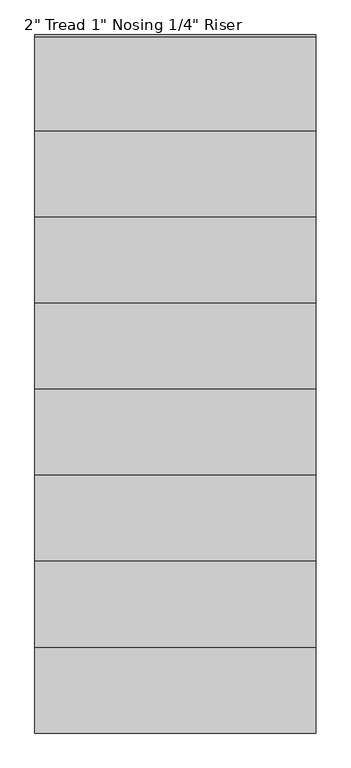
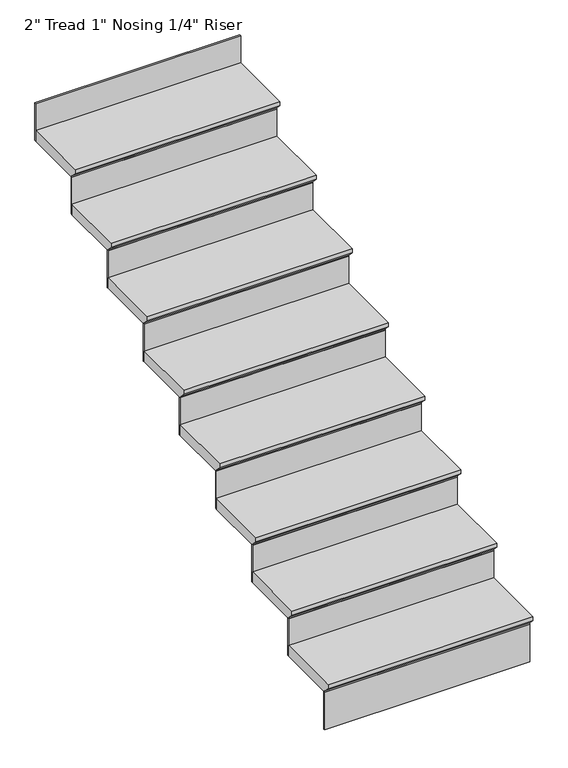
"""IFC4 building model written with IfcOpenShell, lengths in millimetres: stair flight geometry."""

from ifc_helpers import new_model, si_unit, frame, origin, place, context, project, spatial, polyline, outline, extrude, source, transform, mapped, element, save


def stair_flight_b3cbfaaf(model_context):
    return source(origin(), model_context, "Body", "SweptSolid", [
        extrude(outline(polyline([(7893.8147181, 2387.6), (8198.6147181, 2387.6), (8198.6147181, 2336.8), (7919.2147181, 2336.8), (7919.2147181, 2343.15), (7893.8147181, 2368.55), (7893.8147181, 2387.6)])), frame((9078.4923267, 0.0, 0.0), z_axis=(1.0, 0.0, 0.0), x_axis=(0.0, 1.0, 0.0)), (0.0, 0.0, 1.0), 914.4),
        extrude(outline(polyline([(9992.8923267, 7925.5647181), (9992.8923267, 7919.2147181), (9078.4923267, 7919.2147181), (9078.4923267, 7925.5647181), (9992.8923267, 7925.5647181)])), frame((0.0, 0.0, 2159.0), z_axis=(0.0, 0.0, 1.0), x_axis=(1.0, 0.0, 0.0)), (0.0, 0.0, 1.0), 177.8),
        extrude(outline(polyline([(9992.8923267, 8204.9647181), (9992.8923267, 8198.6147181), (9078.4923267, 8198.6147181), (9078.4923267, 8204.9647181), (9992.8923267, 8204.9647181)])), frame((0.0, 0.0, 2336.8), z_axis=(0.0, 0.0, 1.0), x_axis=(1.0, 0.0, 0.0)), (0.0, 0.0, 1.0), 177.8),
        extrude(outline(polyline([(8173.2147181, 2565.4), (8478.0147181, 2565.4), (8478.0147181, 2514.6), (8198.6147181, 2514.6), (8198.6147181, 2520.95), (8173.2147181, 2546.35), (8173.2147181, 2565.4)])), frame((9078.4923267, 0.0, 0.0), z_axis=(1.0, 0.0, 0.0), x_axis=(0.0, 1.0, 0.0)), (0.0, 0.0, 1.0), 914.4),
        extrude(outline(polyline([(9992.8923267, 8484.3647181), (9992.8923267, 8478.0147181), (9078.4923267, 8478.0147181), (9078.4923267, 8484.3647181), (9992.8923267, 8484.3647181)])), frame((0.0, 0.0, 2514.6), z_axis=(0.0, 0.0, 1.0), x_axis=(1.0, 0.0, 0.0)), (0.0, 0.0, 1.0), 177.8),
        extrude(outline(polyline([(8452.6147181, 2743.2), (8757.4147181, 2743.2), (8757.4147181, 2692.4), (8478.0147181, 2692.4), (8478.0147181, 2698.75), (8452.6147181, 2724.15), (8452.6147181, 2743.2)])), frame((9078.4923267, 0.0, 0.0), z_axis=(1.0, 0.0, 0.0), x_axis=(0.0, 1.0, 0.0)), (0.0, 0.0, 1.0), 914.4),
        extrude(outline(polyline([(9992.8923267, 8763.7647181), (9992.8923267, 8757.4147181), (9078.4923267, 8757.4147181), (9078.4923267, 8763.7647181), (9992.8923267, 8763.7647181)])), frame((0.0, 0.0, 2692.4), z_axis=(0.0, 0.0, 1.0), x_axis=(1.0, 0.0, 0.0)), (0.0, 0.0, 1.0), 177.8),
        extrude(outline(polyline([(8732.0147181, 2921.0), (9036.8147181, 2921.0), (9036.8147181, 2870.2), (8757.4147181, 2870.2), (8757.4147181, 2876.55), (8732.0147181, 2901.95), (8732.0147181, 2921.0)])), frame((9078.4923267, 0.0, 0.0), z_axis=(1.0, 0.0, 0.0), x_axis=(0.0, 1.0, 0.0)), (0.0, 0.0, 1.0), 914.4),
        extrude(outline(polyline([(9992.8923267, 9043.1647181), (9992.8923267, 9036.8147181), (9078.4923267, 9036.8147181), (9078.4923267, 9043.1647181), (9992.8923267, 9043.1647181)])), frame((0.0, 0.0, 2870.2), z_axis=(0.0, 0.0, 1.0), x_axis=(1.0, 0.0, 0.0)), (0.0, 0.0, 1.0), 177.8),
        extrude(outline(polyline([(9011.4147181, 3098.8), (9316.2147181, 3098.8), (9316.2147181, 3048.0), (9036.8147181, 3048.0), (9036.8147181, 3054.35), (9011.4147181, 3079.75), (9011.4147181, 3098.8)])), frame((9078.4923267, 0.0, 0.0), z_axis=(1.0, 0.0, 0.0), x_axis=(0.0, 1.0, 0.0)), (0.0, 0.0, 1.0), 914.4),
        extrude(outline(polyline([(9992.8923267, 9322.5647181), (9992.8923267, 9316.2147181), (9078.4923267, 9316.2147181), (9078.4923267, 9322.5647181), (9992.8923267, 9322.5647181)])), frame((0.0, 0.0, 3048.0), z_axis=(0.0, 0.0, 1.0), x_axis=(1.0, 0.0, 0.0)), (0.0, 0.0, 1.0), 177.8),
        extrude(outline(polyline([(9290.8147181, 3276.6), (9595.6147181, 3276.6), (9595.6147181, 3225.8), (9316.2147181, 3225.8), (9316.2147181, 3232.15), (9290.8147181, 3257.55), (9290.8147181, 3276.6)])), frame((9078.4923267, 0.0, 0.0), z_axis=(1.0, 0.0, 0.0), x_axis=(0.0, 1.0, 0.0)), (0.0, 0.0, 1.0), 914.4),
        extrude(outline(polyline([(9992.8923267, 9601.9647181), (9992.8923267, 9595.6147181), (9078.4923267, 9595.6147181), (9078.4923267, 9601.9647181), (9992.8923267, 9601.9647181)])), frame((0.0, 0.0, 3225.8), z_axis=(0.0, 0.0, 1.0), x_axis=(1.0, 0.0, 0.0)), (0.0, 0.0, 1.0), 177.8),
        extrude(outline(polyline([(9570.2147181, 3454.4), (9875.0147181, 3454.4), (9875.0147181, 3403.6), (9595.6147181, 3403.6), (9595.6147181, 3409.95), (9570.2147181, 3435.35), (9570.2147181, 3454.4)])), frame((9078.4923267, 0.0, 0.0), z_axis=(1.0, 0.0, 0.0), x_axis=(0.0, 1.0, 0.0)), (0.0, 0.0, 1.0), 914.4),
        extrude(outline(polyline([(9992.8923267, 9881.3647181), (9992.8923267, 9875.0147181), (9078.4923267, 9875.0147181), (9078.4923267, 9881.3647181), (9992.8923267, 9881.3647181)])), frame((0.0, 0.0, 3403.6), z_axis=(0.0, 0.0, 1.0), x_axis=(1.0, 0.0, 0.0)), (0.0, 0.0, 1.0), 177.8),
        extrude(outline(polyline([(9992.8923267, 10160.7647181), (9992.8923267, 10154.4147181), (9078.4923267, 10154.4147181), (9078.4923267, 10160.7647181), (9992.8923267, 10160.7647181)])), frame((0.0, 0.0, 3581.4), z_axis=(0.0, 0.0, 1.0), x_axis=(1.0, 0.0, 0.0)), (0.0, 0.0, 1.0), 177.8),
        extrude(outline(polyline([(9849.6147181, 3632.2), (10154.4147181, 3632.2), (10154.4147181, 3581.4), (9875.0147181, 3581.4), (9875.0147181, 3587.75), (9849.6147181, 3613.15), (9849.6147181, 3632.2)])), frame((9078.4923267, 0.0, 0.0), z_axis=(1.0, 0.0, 0.0), x_axis=(0.0, 1.0, 0.0)), (0.0, 0.0, 1.0), 914.4),
    ])


if __name__ == "__main__":
    model = new_model("IFC4")
    model_context = context("Model", 3, world=origin())
    ifc_project = project(units=[si_unit("LENGTHUNIT", "METRE", prefix="MILLI")], contexts=[model_context])
    site = spatial("IfcSite", under=ifc_project)
    building = spatial("IfcBuilding", under=site)
    placement = place(None, origin())
    stair_flight_shape = stair_flight_b3cbfaaf(model_context)
    element("IfcStairFlight", 1, ObjectType="2\" Tread 1\" Nosing 1/4\" Riser", at=placement, inside=building, context=model_context, shape_type="MappedRepresentation", body=[
        mapped(stair_flight_shape, transform((0.0, 0.0, 0.0), x_axis=(1.0, 0.0, 0.0), y_axis=(0.0, 1.0, 0.0), z_axis=(0.0, 0.0, 1.0))),
    ])
    save(model, "model.ifc")
